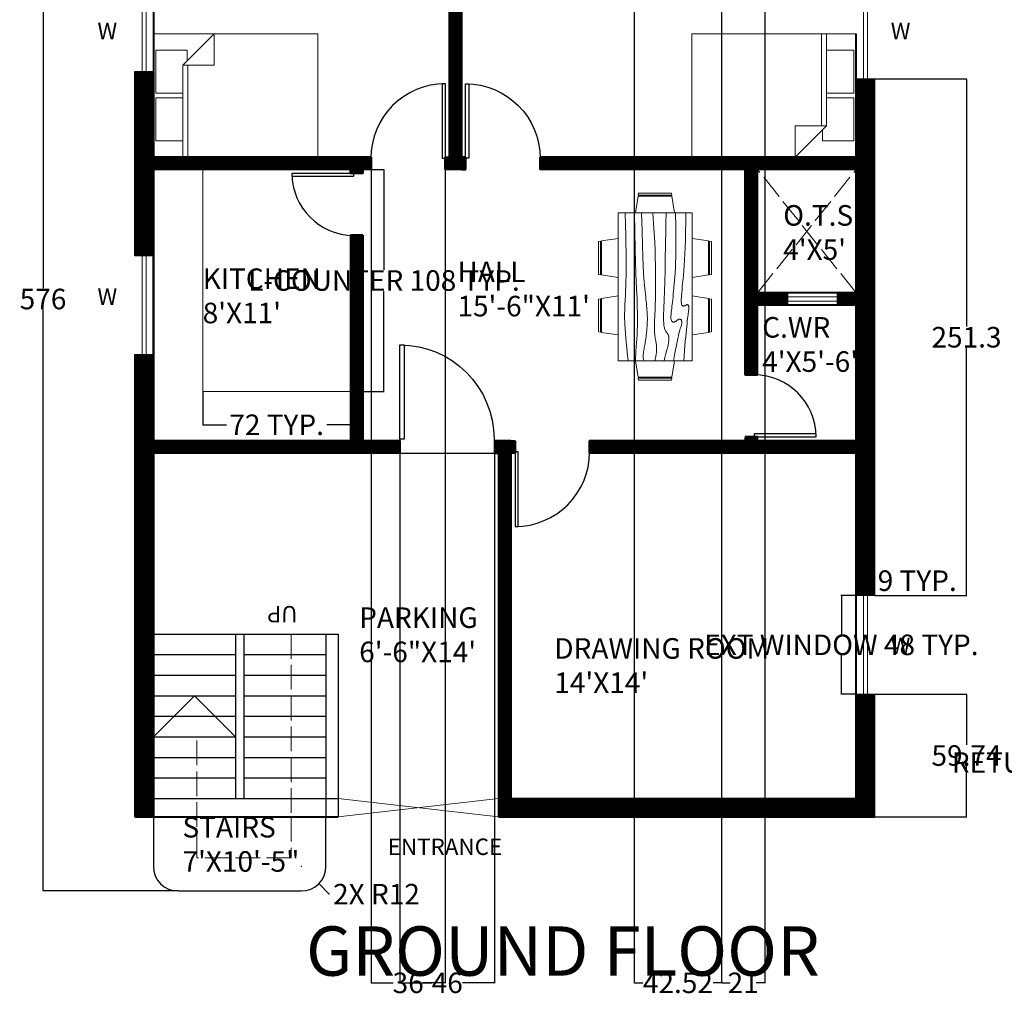
# Model space of a CAD drawing. Units: inches. Extents: x 345 to 1363, y 285 to 1014.
# Tile 1 of 4: x 345 to 824, y 285 to 760. Entities that reach past the tile are written whole.
import ezdxf

# ---------------------------------------------------------------- set-up
doc = ezdxf.new("R2010")
doc.units = ezdxf.units.IN
doc.header["$MEASUREMENT"] = 0
doc.linetypes.add('ACAD_ISO02W100', pattern=[15, 12, -3])
for name, color, linetype, lineweight in [('A-ANNO-DIMS', 2, 'Continuous', 18), ('A-ANNO-SYMB', 3, 'Continuous', 18), ('A-ANNO-TEXT', 7, 'Continuous', 18), ('A-ANNO-TITL', 7, 'Continuous', 35), ('A-AREA-IDEN', 7, 'Continuous', 18), ('A-FLOR-CASE', 8, 'Continuous', 18), ('A-FLOR-OPEN', 8, 'Continuous', 18), ('A-FLOR-OPEN-OVHD', 8, 'ACAD_ISO02W100', 13), ('A-FLOR-STRS', 7, 'Continuous', 25), ('A-FLOR-STRS-PATH', 3, 'ACAD_ISO02W100', 18), ('A-FURN', 9, 'Continuous', 18), ('A-GLAZ', 4, 'Continuous', 18), ('A-WALL', 7, 'Continuous', 40), ('A-WALL-PATT', 252, 'Continuous', 9), ('BED', 9, 'Continuous', 18), ('DOOR', 4, 'Continuous', 25)]:
    doc.layers.add(name, color=color, linetype=linetype, lineweight=lineweight)
doc.styles.get("Standard").update_dxf_attribs({"font": 'arial.ttf'})
doc.dimstyles.get("Standard").update_dxf_attribs({"dimtxt": 10, "dimasz": 0.18, "dimexe": 0.18, "dimexo": 0.0625, "dimgap": 0.09, "dimtad": 0, "dimtih": 1, "dimtoh": 1, "dimdec": 0, "dimzin": 0, "dimdsep": 46, "dimlunit": 3, "dimtxsty": 'Standard', "dimcen": 0.09, "dimadec": 0, "dimazin": 0, "dimtfac": 1, "dimtdec": 0, "dimtofl": 0, "dimtmove": 0, "dimatfit": 3, "dimfxl": 1, "dimtolj": 1, "dimtzin": 0, "dimarcsym": 0})

# ---------------------------------------------------------------- blocks, each defined once
blk = doc.blocks.new('Bed - Queen')
for p, q in [((0, -80.00003), (0, 0)), ((0, 0), (59.99999, 0)), ((59.99999, 0), (59.99999, -80.00003)), ((7.99999, -1.2), (28.79998, -1.2)), ((7.99999, -14.4), (7.99999, -1.2)), ((28.79998, -1.2), (28.79998, -14.4)), ((31.19999, -1.2), (51.99999, -1.2)), ((31.19999, -14.4), (31.19999, -1.2)), ((51.99999, -1.2), (51.99999, -16.4)), ((0, -14.4), (44.8, -14.4)), ((44.8, -16.8), (0, -16.8)), ((59.99999, -29.6), (44.8, -14.4)), ((44.8, -14.4), (44.8, -29.6)), ((51.99999, -16.4), (46.79936, -16.4)), ((44.8, -29.6), (59.99999, -29.6)), ((59.99999, -80.00003), (0, -80.00003))]:
    blk.add_line(p, q)
blk = doc.blocks.new('Dining Set - 36 x 72 in.')
for p, q in [((-22.2343, 26.00059), (-23.4847, 17.99762)), ((-22.2304, 26), (-5.7608, 26)), ((-22, 27.5), (-22.1562, 26.50042)), ((-5.8416, 26.5), (-22.1534, 26.5)), ((-22, 27.5), (-6, 27.5)), ((-5.8437, 26.49966), (-6, 27.5)), ((-4.5152, 17.99762), (-5.7655, 25.99926)), ((5.7657, 26.00059), (4.5153, 17.99762)), ((5.7696, 26), (22.2392, 26)), ((6, 27.5), (5.8438, 26.50042)), ((22.1584, 26.5), (5.8466, 26.5)), ((6, 27.5), (22, 27.5)), ((22.1563, 26.49966), (22, 27.5)), ((23.4848, 17.99762), (22.2345, 25.99926)), ((36, 18), (-36, 18)), ((-36, 18), (-36, -18)), ((36, -18), (36, 18)), ((-45.5, 8), (-44.5004, 8.15617)), ((-45.5, 8), (-45.5, -8)), ((-44.5, -8.15843), (-44.5, 8.15338)), ((-44.0006, 8.23428), (-35.9976, 9.48474)), ((-44, 8.23041), (-44, -8.23915)), ((44.0006, 8.23428), (35.9976, 9.48474)), ((44, 8.23041), (44, -8.23915)), ((44.5, -8.15843), (44.5, 8.15338)), ((45.5, 8), (44.5005, 8.15617)), ((45.5, 8), (45.5, -8)), ((-44.4997, -8.15631), (-45.5, -8)), ((-35.9976, -9.48476), (-43.9993, -8.2345)), ((35.9976, -9.48476), (43.9993, -8.2345)), ((44.4997, -8.15631), (45.5, -8)), ((-36, -18), (36, -18)), ((-22.2343, -26.0006), (-23.4847, -17.99762)), ((-4.5152, -17.99762), (-5.7655, -25.99928)), ((5.7657, -26.0006), (4.5153, -17.99762)), ((23.4848, -17.99762), (22.2345, -25.99928)), ((-22.2304, -26), (-5.7608, -26)), ((-22, -27.5), (-22.1562, -26.50044)), ((-5.8416, -26.5), (-22.1534, -26.5)), ((-22, -27.5), (-6, -27.5)), ((-5.8437, -26.49967), (-6, -27.5)), ((5.7696, -26), (22.2392, -26)), ((6, -27.5), (5.8438, -26.50044)), ((22.1584, -26.5), (5.8466, -26.5)), ((6, -27.5), (22, -27.5)), ((22.1563, -26.49967), (22, -27.5))]:
    blk.add_line(p, q)
for points in [[(-36, 15), (-31.1772, 14.97754), (-26.8079, 14.91406), (-22.8538, 14.81543), (-19.276, 14.6875), (-16.0362, 14.53613), (-13.0957, 14.36718), (-10.4159, 14.18652), (-7.9583, 14), (-5.6904, 13.81315), (-3.6035, 13.63021), (-1.6954, 13.45508), (0.0365, 13.29166), (1.5945, 13.14388), (2.9811, 13.01562), (4.1988, 12.9108), (5.25, 12.83333), (6.1393, 12.78613), (6.8802, 12.76823), (7.4883, 12.77767), (7.9792, 12.8125), (8.3685, 12.87077), (8.6719, 12.95052), (8.9049, 13.0498), (9.0833, 13.16666), (9.2205, 13.29899), (9.3216, 13.44401), (9.3895, 13.59879), (9.4271, 13.76041), (9.4373, 13.92594), (9.4232, 14.09245), (9.3875, 14.257), (9.3333, 14.41666), (9.2638, 14.56917), (9.1836, 14.71484), (9.0975, 14.85465), (9.0104, 14.98958), (8.9272, 15.1206), (8.8529, 15.2487), (8.7922, 15.37483), (8.75, 15.5), (8.7305, 15.62467), (8.7344, 15.74739), (8.7617, 15.86621), (8.8125, 15.97916), (8.8867, 16.08431), (8.9844, 16.17968), (9.1055, 16.26334), (9.25, 16.33333), (9.4189, 16.38802), (9.6172, 16.42708), (9.8506, 16.45052), (10.125, 16.45833), (10.4463, 16.45052), (10.8203, 16.42708), (11.2529, 16.38802), (11.75, 16.33333), (12.3184, 16.26318), (12.9694, 16.17838), (13.7151, 16.07991), (14.5677, 15.96875), (15.5395, 15.84586), (16.6426, 15.71224), (17.8893, 15.56884), (19.2917, 15.41666), (20.859, 15.25667), (22.5879, 15.08984), (24.4721, 14.91715), (26.5052, 14.73958), (28.6809, 14.5581), (30.9929, 14.3737), (33.4347, 14.18733), (36, 14)], [(-36, 10), (-28.9766, 10.14274), (-23.1725, 10.20442), (-18.4241, 10.19775), (-14.5677, 10.13541), (-11.4399, 10.03011), (-8.877, 9.89453), (-6.7154, 9.74137), (-4.7917, 9.58333), (-2.9698, 9.43082), (-1.2246, 9.28515), (0.4415, 9.14534), (2.026, 9.01041), (3.5266, 8.87939), (4.9408, 8.7513), (6.266, 8.62516), (7.5, 8.5), (8.6411, 8.37549), (9.6914, 8.2539), (10.6538, 8.13818), (11.5312, 8.03125), (12.3267, 7.93603), (13.043, 7.85547), (13.6831, 7.79248), (14.25, 7.75), (14.7471, 7.7303), (15.1797, 7.73307), (15.5537, 7.75732), (15.875, 7.80208), (16.1494, 7.86637), (16.3828, 7.94922), (16.5811, 8.04964), (16.75, 8.16666), (16.8944, 8.29915), (17.0143, 8.44531), (17.1089, 8.60319), (17.1771, 8.77083), (17.218, 8.94629), (17.2305, 9.1276), (17.2137, 9.31282), (17.1667, 9.5), (17.0895, 9.6875), (16.987, 9.875), (16.8649, 10.0625), (16.7292, 10.25), (16.5856, 10.4375), (16.4401, 10.625), (16.2985, 10.8125), (16.1667, 11), (16.05, 11.18733), (15.9518, 11.3737), (15.8752, 11.5581), (15.8229, 11.73958), (15.798, 11.91715), (15.8034, 12.08984), (15.842, 12.25667), (15.9167, 12.41666), (16.0295, 12.56836), (16.1784, 12.70833), (16.3605, 12.83268), (16.5729, 12.9375), (16.8127, 13.01888), (17.0768, 13.07291), (17.3625, 13.0957), (17.6667, 13.08333), (17.9894, 13.03312), (18.3418, 12.94726), (18.7382, 12.82918), (19.1927, 12.68229), (19.7195, 12.51001), (20.3327, 12.31575), (21.0465, 12.10294), (21.875, 11.875), (22.8357, 11.63354), (23.959, 11.37304), (25.2786, 11.08618), (26.8282, 10.76562), (28.6414, 10.40405), (30.752, 9.99414), (33.1936, 9.52856), (36, 9)], [(-36, 5.5), (-30.7157, 5.3348), (-26.069, 5.20963), (-21.9946, 5.11767), (-18.4271, 5.05208), (-15.3009, 5.00602), (-12.5508, 4.97265), (-10.1112, 4.94515), (-7.9167, 4.91666), (-5.909, 4.88167), (-4.0586, 4.83984), (-2.3429, 4.79215), (-0.7396, 4.73958), (0.7739, 4.6831), (2.22, 4.6237), (3.6213, 4.56233), (5, 4.5), (6.373, 4.43782), (7.7344, 4.3776), (9.0723, 4.32129), (10.375, 4.27083), (11.6309, 4.22819), (12.8281, 4.19531), (13.9551, 4.17415), (15, 4.16666), (15.954, 4.17448), (16.819, 4.19791), (17.6001, 4.23698), (18.3021, 4.29166), (18.9299, 4.36198), (19.4883, 4.44791), (19.9823, 4.54948), (20.4167, 4.66666), (20.7969, 4.79899), (21.1302, 4.94401), (21.4245, 5.09879), (21.6875, 5.26041), (21.9271, 5.42594), (22.1511, 5.59245), (22.3672, 5.757), (22.5834, 5.91666), (22.8065, 6.06868), (23.0404, 6.21093), (23.2879, 6.34147), (23.5521, 6.45833), (23.8358, 6.55957), (24.142, 6.64323), (24.4735, 6.70735), (24.8334, 6.75), (25.2235, 6.76969), (25.642, 6.76692), (26.0858, 6.74267), (26.5521, 6.69791), (27.0379, 6.63362), (27.5404, 6.55078), (28.0565, 6.45036), (28.5834, 6.33333), (29.1242, 6.19987), (29.7071, 6.04687), (30.3661, 5.87044), (31.1354, 5.66666), (32.0493, 5.43164), (33.142, 5.16146), (34.4475, 4.85221), (36, 4.5)], [(-36, -1), (-30.7915, -0.6591), (-26.0195, -0.38216), (-21.6519, -0.16284), (-17.6563, 0.00521), (-14.0005, 0.12833), (-10.6523, 0.21289), (-7.5796, 0.26522), (-4.75, 0.29166), (-2.134, 0.29793), (0.2878, 0.28711), (2.5317, 0.26163), (4.6146, 0.22396), (6.5529, 0.17651), (8.3633, 0.12174), (10.0623, 0.06209), (11.6667, 0), (13.1899, -0.06201), (14.6341, -0.1211), (15.9982, -0.17432), (17.2813, -0.21875), (18.4823, -0.25147), (19.6003, -0.26953), (20.6343, -0.27002), (21.5834, -0.25), (22.4481, -0.20768), (23.2357, -0.14584), (23.9549, -0.06836), (24.6146, 0.02083), (25.2235, 0.11784), (25.7904, 0.21875), (26.3241, 0.31966), (26.8334, 0.41666), (27.3265, 0.50618), (27.8099, 0.58593), (28.2894, 0.65397), (28.7709, 0.70833), (29.2601, 0.74707), (29.763, 0.76823), (30.2855, 0.76985), (30.8334, 0.75), (31.4088, 0.70784), (31.9994, 0.64713), (32.589, 0.57275), (33.1615, 0.48958), (33.7008, 0.4025), (34.1908, 0.3164), (34.6153, 0.23616), (34.9584, 0.16666), (35.2099, 0.11165), (35.3848, 0.07031), (35.504, 0.04069), (35.5886, 0.02083), (35.6594, 0.00879), (35.7377, 0.0026), (35.8442, 0.00032), (36, 0)], [(-36, -6.5), (-27.1843, -6.31267), (-20.084, -6.1263), (-14.469, -5.9419), (-10.1094, -5.76042), (-6.7752, -5.58285), (-4.2363, -5.41016), (-2.2629, -5.24333), (-0.625, -5.08334), (0.8708, -4.93099), (2.2715, -4.78646), (3.5872, -4.64974), (4.8281, -4.52084), (6.0046, -4.39974), (7.127, -4.28646), (8.2053, -4.18099), (9.25, -4.08334), (10.2705, -3.99382), (11.2734, -3.91407), (12.2647, -3.84603), (13.25, -3.79167), (14.2354, -3.75293), (15.2266, -3.73177), (16.2295, -3.73015), (17.25, -3.75), (18.2912, -3.79248), (19.3451, -3.85547), (20.4009, -3.93604), (21.4479, -4.03125), (22.4754, -4.13819), (23.4727, -4.25391), (24.4289, -4.37549), (25.3334, -4.5), (26.1785, -4.62492), (26.9694, -4.74935), (27.7145, -4.87281), (28.4219, -4.99479), (29.1, -5.11483), (29.7572, -5.23242), (30.4016, -5.34709), (31.0417, -5.45834), (31.6837, -5.56437), (32.3262, -5.65821), (32.9658, -5.73153), (33.599, -5.77604), (34.2224, -5.78345), (34.8327, -5.74545), (35.4264, -5.65373), (36, -5.5)], [(-36, -10), (-26.4022, -9.81299), (-18.4675, -9.62891), (-11.9839, -9.45069), (-6.7396, -9.28125), (-2.5226, -9.12354), (0.8789, -8.98047), (3.6769, -8.85498), (6.0833, -8.75), (8.2767, -8.66765), (10.3021, -8.60677), (12.1712, -8.56543), (13.8958, -8.54167), (15.4876, -8.53353), (16.9583, -8.53907), (18.3197, -8.55632), (19.5834, -8.58334), (20.7616, -8.61841), (21.8685, -8.66081), (22.9188, -8.71004), (23.9271, -8.76563), (24.9081, -8.82707), (25.8763, -8.89388), (26.8465, -8.96558), (27.8334, -9.04167), (28.8474, -9.12118), (29.8828, -9.20117), (30.93, -9.27824), (31.9792, -9.34896), (33.0205, -9.40991), (34.0443, -9.45768), (35.0407, -9.48885), (36, -9.5)], [(-36, -14.5), (-30.0881, -14.33513), (-25.0332, -14.21224), (-20.7312, -14.12647), (-17.0781, -14.07292), (-13.97, -14.04671), (-11.3027, -14.04297), (-8.9724, -14.05681), (-6.875, -14.08334), (-4.9224, -14.11833), (-3.0905, -14.16016), (-1.3709, -14.20785), (0.2448, -14.26042), (1.7647, -14.3169), (3.1973, -14.3763), (4.5507, -14.43767), (5.8333, -14.5), (7.0554, -14.5621), (8.235, -14.62175), (9.3922, -14.67652), (10.5469, -14.72396), (11.7192, -14.76164), (12.929, -14.78711), (14.1965, -14.79794), (15.5417, -14.79167), (16.9933, -14.76424), (18.6152, -14.70508), (20.4804, -14.60197), (22.6615, -14.44271), (25.2312, -14.21509), (28.2624, -13.9069), (31.8277, -13.50594), (36, -13)]]:
    blk.add_lwpolyline(points)
blk = doc.blocks.new('*U8')
for p, q in [((0, 0), (0, -6)), ((-40, 0), (-40, -6))]:
    blk.add_line(p, q)
blk.add_lwpolyline([(0, 0), (0, 40), (-1.75, 40), (-1.75, 0)], close=True)
blk.add_arc((0, 0), 40, 90, 180)
blk = doc.blocks.new('*U9')
for p, q in [((0, 0), (0, 6)), ((40, 0), (40, 6))]:
    blk.add_line(p, q)
blk.add_lwpolyline([(0, 0), (0, -40), (1.75, -40), (1.75, 0)], close=True)
blk.add_arc((0, 0), 40, 270, 360)
blk = doc.blocks.new('WIN-48IN-EXT')
for p, q in [((9, 48), (0, 48)), ((3.5, 0), (3.5, 48)), ((5.5, 0), (5.5, 48)), ((9, 0), (0, 0))]:
    blk.add_line(p, q)
blk = doc.blocks.new('WIN-24IN-VENT')
for p, q in [((0, 24), (6, 24)), ((2, 24), (2, 0)), ((4, 24), (4, 0)), ((0, 0), (6, 0))]:
    blk.add_line(p, q)
blk = doc.blocks.new('KITCHEN-L-COUNTER')
for p in [(0, 108), (72, 0)]:
    blk.add_line(p, (0, 0))
blk = doc.blocks.new('STAIR-RETURN-84IN')
for p, q in [((0, 89), (44, 89)), ((40, 89), (40, 9)), ((44, 89), (44, 9)), ((44, 89), (90, 89)), ((84, 89), (84, 0)), ((90, 89), (90, 0)), ((0, 79), (40, 79)), ((44, 79), (84, 79)), ((0, 69), (40, 69)), ((44, 69), (84, 69)), ((0, 59), (40, 59)), ((44, 59), (84, 59)), ((0, 49), (40, 49)), ((44, 49), (84, 49)), ((0, 39), (40, 39)), ((44, 39), (84, 39)), ((0, 29), (40, 29)), ((44, 29), (84, 29)), ((0, 19), (40, 19)), ((44, 19), (84, 19)), ((0, 9), (90, 9)), ((0, 0), (0, -24)), ((84, -24), (84, 0)), ((12, -36), (72, -36))]:
    blk.add_line(p, q)
for centre, start, end in [((12, -24), 180, 270), ((72, -24), 270, 0)]:
    blk.add_arc(centre, 12, start, end)
blk = doc.blocks.new('STAIR-DIRECTION-ARROWHEAD')
for p, q in [((-20, 0), (0, 20)), ((0, 20), (20, 0)), ((0, 0), (-20, 0)), ((20, 0), (1.17, 0))]:
    blk.add_line(p, q)
blk = doc.blocks.new('*D16')
at = {"layer": 'A-ANNO-DIMS', "color": 0, "lineweight": -2, "transparency": 16777216}
for p, q in [((751.9, 479.51), (744.59, 479.51)), ((744.77, 479.33), (744.77, 460.77)), ((744.77, 431.69), (744.77, 450.24)), ((751.9, 431.51), (744.59, 431.51))]:
    blk.add_line(p, q, dxfattribs=at)
at = {"layer": 'A-ANNO-DIMS', "color": 0, "transparency": 16777216}
for points in [[(744.74, 479.33), (744.8, 479.33), (744.77, 479.51)], [(744.74, 431.69), (744.8, 431.69), (744.77, 431.51)]]:
    blk.add_solid(points, dxfattribs=at)
at = {"layer": 'Defpoints', "color": 0, "transparency": 16777216}
for p in [(744.77, 479.51), (751.97, 479.51), (751.97, 431.51)]:
    blk.add_point(p, dxfattribs=at)
at = {"layer": 'A-ANNO-DIMS', "color": 0, "transparency": 16777216, "insert": (744.77, 455.51), "char_height": 10, "attachment_point": 5}
blk.add_mtext('\\A1;EXT WINDOW 48 TYP.', dxfattribs=at)
blk = doc.blocks.new('*D17')
at = {"layer": 'A-ANNO-DIMS', "color": 0, "lineweight": -2, "transparency": 16777216}
for p, q in [((751.97, 479.57), (751.97, 486.89)), ((752.15, 486.71), (760.79, 486.71)), ((760.97, 479.57), (760.97, 486.89)), ((760.97, 486.71), (761.15, 486.71))]:
    blk.add_line(p, q, dxfattribs=at)
at = {"layer": 'A-ANNO-DIMS', "color": 0, "transparency": 16777216}
for points in [[(752.15, 486.74), (752.15, 486.68), (751.97, 486.71)], [(760.79, 486.74), (760.79, 486.68), (760.97, 486.71)]]:
    blk.add_solid(points, dxfattribs=at)
at = {"layer": 'Defpoints', "color": 0, "transparency": 16777216}
for p in [(760.97, 486.71), (751.97, 479.51), (760.97, 479.51)]:
    blk.add_point(p, dxfattribs=at)
at = {"layer": 'A-ANNO-DIMS', "color": 0, "transparency": 16777216, "insert": (781.69, 486.71), "char_height": 10, "attachment_point": 5}
blk.add_mtext('\\A1;9 TYP.', dxfattribs=at)
blk = doc.blocks.new('*D26')
at = {"layer": 'A-ANNO-DIMS', "color": 0, "lineweight": -2, "transparency": 16777216}
for p, q in [((506.03, 686.76), (522.35, 686.76)), ((522.17, 686.58), (522.17, 638.03)), ((522.17, 578.94), (522.17, 627.5)), ((506.03, 578.76), (522.35, 578.76))]:
    blk.add_line(p, q, dxfattribs=at)
at = {"layer": 'A-ANNO-DIMS', "color": 0, "transparency": 16777216}
for points in [[(522.14, 686.58), (522.2, 686.58), (522.17, 686.76)], [(522.14, 578.94), (522.2, 578.94), (522.17, 578.76)]]:
    blk.add_solid(points, dxfattribs=at)
at = {"layer": 'Defpoints', "color": 0, "transparency": 16777216}
for p in [(505.97, 686.76), (522.17, 686.76), (505.97, 578.76)]:
    blk.add_point(p, dxfattribs=at)
at = {"layer": 'A-ANNO-DIMS', "color": 0, "transparency": 16777216, "insert": (522.17, 632.76), "char_height": 10, "attachment_point": 5}
blk.add_mtext('\\A1;L-COUNTER 108 TYP.', dxfattribs=at)
blk = doc.blocks.new('*D27')
at = {"layer": 'A-ANNO-DIMS', "color": 0, "lineweight": -2, "transparency": 16777216}
for p, q in [((433.97, 578.7), (433.97, 562.38)), ((505.97, 578.7), (505.97, 562.38)), ((434.15, 562.56), (445.58, 562.56)), ((505.79, 562.56), (494.35, 562.56))]:
    blk.add_line(p, q, dxfattribs=at)
at = {"layer": 'A-ANNO-DIMS', "color": 0, "transparency": 16777216}
for points in [[(434.15, 562.59), (434.15, 562.53), (433.97, 562.56)], [(505.79, 562.59), (505.79, 562.53), (505.97, 562.56)]]:
    blk.add_solid(points, dxfattribs=at)
at = {"layer": 'Defpoints', "color": 0, "transparency": 16777216}
for p in [(433.97, 578.76), (505.97, 578.76), (505.97, 562.56)]:
    blk.add_point(p, dxfattribs=at)
at = {"layer": 'A-ANNO-DIMS', "color": 0, "transparency": 16777216, "insert": (469.97, 562.56), "char_height": 10, "attachment_point": 5}
blk.add_mtext('\\A1;72 TYP.', dxfattribs=at)
blk = doc.blocks.new('*D28')
at = {"layer": 'A-ANNO-DIMS', "color": 0, "lineweight": -2, "transparency": 16777216}
for p, q in [((892.32, 460.76), (873.45, 460.76)), ((873.63, 460.58), (873.63, 403.52)), ((873.63, 335.94), (873.63, 393)), ((892.32, 335.76), (873.45, 335.76))]:
    blk.add_line(p, q, dxfattribs=at)
at = {"layer": 'A-ANNO-DIMS', "color": 0, "transparency": 16777216}
for points in [[(873.6, 460.58), (873.66, 460.58), (873.63, 460.76)], [(873.6, 335.94), (873.66, 335.94), (873.63, 335.76)]]:
    blk.add_solid(points, dxfattribs=at)
at = {"layer": 'Defpoints', "color": 0, "transparency": 16777216}
for p in [(873.63, 460.76), (892.38, 460.76), (892.38, 335.76)]:
    blk.add_point(p, dxfattribs=at)
at = {"layer": 'A-ANNO-DIMS', "color": 0, "transparency": 16777216, "insert": (873.63, 398.26), "char_height": 10, "attachment_point": 5}
blk.add_mtext('\\A1;RETURN STAIR 125 TYP.', dxfattribs=at)
blk = doc.blocks.new('*D31')
at = {"layer": 'A-ANNO-DIMS', "color": 0, "lineweight": -2, "transparency": 16777216}
for p, q in [((400.9, 911.76), (356.09, 911.76)), ((356.27, 911.58), (356.27, 628.96)), ((356.27, 335.94), (356.27, 618.57)), ((421.9, 335.76), (356.09, 335.76))]:
    blk.add_line(p, q, dxfattribs=at)
at = {"layer": 'A-ANNO-DIMS', "color": 0, "transparency": 16777216}
for points in [[(356.24, 911.58), (356.3, 911.58), (356.27, 911.76)], [(356.24, 335.94), (356.3, 335.94), (356.27, 335.76)]]:
    blk.add_solid(points, dxfattribs=at)
at = {"layer": 'Defpoints', "color": 0, "transparency": 16777216}
for p in [(356.27, 911.76), (400.97, 911.76), (421.97, 335.76)]:
    blk.add_point(p, dxfattribs=at)
at = {"layer": 'A-ANNO-DIMS', "color": 0, "transparency": 16777216, "insert": (356.27, 623.76), "char_height": 10, "attachment_point": 5}
blk.add_mtext('\\A1;576', dxfattribs=at)
blk = doc.blocks.new('*D37')
at = {"layer": 'A-ANNO-DIMS', "color": 0, "lineweight": -2, "transparency": 16777216}
for p, q in [((761.03, 431.51), (805.85, 431.51)), ((805.67, 431.33), (805.67, 406.83)), ((805.67, 371.94), (805.67, 396.44)), ((761.03, 371.76), (805.85, 371.76))]:
    blk.add_line(p, q, dxfattribs=at)
at = {"layer": 'A-ANNO-DIMS', "color": 0, "transparency": 16777216}
for points in [[(805.64, 431.33), (805.7, 431.33), (805.67, 431.51)], [(805.64, 371.94), (805.7, 371.94), (805.67, 371.76)]]:
    blk.add_solid(points, dxfattribs=at)
at = {"layer": 'Defpoints', "color": 0, "transparency": 16777216}
for p in [(760.97, 431.51), (760.97, 371.76), (805.67, 371.76)]:
    blk.add_point(p, dxfattribs=at)
at = {"layer": 'A-ANNO-DIMS', "color": 0, "transparency": 16777216, "insert": (805.67, 401.64), "char_height": 10, "attachment_point": 5}
blk.add_mtext('\\A1;59.74', dxfattribs=at)
blk = doc.blocks.new('*D38')
at = {"layer": 'A-ANNO-DIMS', "color": 0, "lineweight": -2, "transparency": 16777216}
for p, q in [((761.03, 730.81), (805.85, 730.81)), ((805.67, 730.63), (805.67, 610.36)), ((805.67, 479.69), (805.67, 599.96)), ((761.03, 479.51), (805.85, 479.51))]:
    blk.add_line(p, q, dxfattribs=at)
at = {"layer": 'A-ANNO-DIMS', "color": 0, "transparency": 16777216}
for points in [[(805.64, 730.63), (805.7, 730.63), (805.67, 730.81)], [(805.64, 479.69), (805.7, 479.69), (805.67, 479.51)]]:
    blk.add_solid(points, dxfattribs=at)
at = {"layer": 'Defpoints', "color": 0, "transparency": 16777216}
for p in [(760.97, 730.81), (760.97, 479.51), (805.67, 479.51)]:
    blk.add_point(p, dxfattribs=at)
at = {"layer": 'A-ANNO-DIMS', "color": 0, "transparency": 16777216, "insert": (805.67, 605.16), "char_height": 10, "attachment_point": 5}
blk.add_mtext('\\A1;251.3', dxfattribs=at)
blk = doc.blocks.new('*D39')
at = {"layer": 'A-ANNO-DIMS', "color": 0, "lineweight": -2, "transparency": 16777216}
for p, q in [((529.97, 548.7), (529.97, 290.88)), ((575.97, 548.7), (575.97, 290.88)), ((530.15, 291.06), (545.52, 291.06)), ((575.79, 291.06), (560.42, 291.06))]:
    blk.add_line(p, q, dxfattribs=at)
at = {"layer": 'A-ANNO-DIMS', "color": 0, "transparency": 16777216}
for points in [[(530.15, 291.09), (530.15, 291.03), (529.97, 291.06)], [(575.79, 291.09), (575.79, 291.03), (575.97, 291.06)]]:
    blk.add_solid(points, dxfattribs=at)
at = {"layer": 'Defpoints', "color": 0, "transparency": 16777216}
for p in [(529.97, 548.76), (575.97, 548.76), (575.97, 291.06)]:
    blk.add_point(p, dxfattribs=at)
at = {"layer": 'A-ANNO-DIMS', "color": 0, "transparency": 16777216, "insert": (552.97, 291.06), "char_height": 10, "attachment_point": 5}
blk.add_mtext('\\A1;46', dxfattribs=at)
blk = doc.blocks.new('*D40')
at = {"layer": 'A-ANNO-DIMS', "color": 0, "lineweight": -2, "transparency": 16777216}
for p, q in [((515.97, 686.7), (515.97, 290.88)), ((551.97, 686.7), (551.97, 290.88)), ((516.15, 291.06), (526.72, 291.06)), ((551.79, 291.06), (541.21, 291.06))]:
    blk.add_line(p, q, dxfattribs=at)
at = {"layer": 'A-ANNO-DIMS', "color": 0, "transparency": 16777216}
for points in [[(516.15, 291.09), (516.15, 291.03), (515.97, 291.06)], [(551.79, 291.09), (551.79, 291.03), (551.97, 291.06)]]:
    blk.add_solid(points, dxfattribs=at)
at = {"layer": 'Defpoints', "color": 0, "transparency": 16777216}
for p in [(515.97, 686.76), (551.97, 686.76), (551.97, 291.06)]:
    blk.add_point(p, dxfattribs=at)
at = {"layer": 'A-ANNO-DIMS', "color": 0, "transparency": 16777216, "insert": (533.97, 291.06), "char_height": 10, "attachment_point": 5}
blk.add_mtext('\\A1;36', dxfattribs=at)
blk = doc.blocks.new('*D43')
at = {"layer": 'A-ANNO-DIMS', "color": 0, "lineweight": -2, "transparency": 16777216}
for p, q in [((643.97, 902.7), (643.97, 290.88)), ((686.49, 894.7), (686.49, 290.88)), ((644.15, 291.06), (648.11, 291.06)), ((686.31, 291.06), (682.34, 291.06))]:
    blk.add_line(p, q, dxfattribs=at)
at = {"layer": 'A-ANNO-DIMS', "color": 0, "transparency": 16777216}
for points in [[(644.15, 291.09), (644.15, 291.03), (643.97, 291.06)], [(686.31, 291.09), (686.31, 291.03), (686.49, 291.06)]]:
    blk.add_solid(points, dxfattribs=at)
at = {"layer": 'Defpoints', "color": 0, "transparency": 16777216}
for p in [(643.97, 902.76), (686.49, 894.76), (686.49, 291.06)]:
    blk.add_point(p, dxfattribs=at)
at = {"layer": 'A-ANNO-DIMS', "color": 0, "transparency": 16777216, "insert": (665.23, 291.06), "char_height": 10, "attachment_point": 5}
blk.add_mtext('\\A1;42.52', dxfattribs=at)
blk = doc.blocks.new('*D44')
at = {"layer": 'A-ANNO-DIMS', "color": 0, "lineweight": -2, "transparency": 16777216}
for p, q in [((686.49, 894.7), (686.49, 290.88)), ((707.49, 894.7), (707.49, 290.88)), ((686.67, 291.06), (690.61, 291.06)), ((707.31, 291.06), (703.36, 291.06))]:
    blk.add_line(p, q, dxfattribs=at)
at = {"layer": 'A-ANNO-DIMS', "color": 0, "transparency": 16777216}
for points in [[(686.67, 291.09), (686.67, 291.03), (686.49, 291.06)], [(707.31, 291.09), (707.31, 291.03), (707.49, 291.06)]]:
    blk.add_solid(points, dxfattribs=at)
at = {"layer": 'Defpoints', "color": 0, "transparency": 16777216}
for p in [(686.49, 894.76), (707.49, 894.76), (707.49, 291.06)]:
    blk.add_point(p, dxfattribs=at)
at = {"layer": 'A-ANNO-DIMS', "color": 0, "transparency": 16777216, "insert": (696.99, 291.06), "char_height": 10, "attachment_point": 5}
blk.add_mtext('\\A1;21', dxfattribs=at)
blk = doc.blocks.new('*D47')
at = {"layer": 'A-ANNO-DIMS', "color": 0, "lineweight": -2, "transparency": 16777216}
for p, q in [((481.88, 347.76), (482.06, 347.76)), ((481.97, 347.67), (481.97, 347.85)), ((495.54, 334.19), (490.58, 339.15)), ((495.72, 334.19), (495.54, 334.19))]:
    blk.add_line(p, q, dxfattribs=at)
at = {"layer": 'A-ANNO-DIMS', "color": 0, "transparency": 16777216}
blk.add_solid([(490.6, 339.17), (490.56, 339.13), (490.45, 339.28)], dxfattribs=at)
at = {"layer": 'Defpoints', "color": 0, "transparency": 16777216}
for p in [(481.97, 347.76), (490.45, 339.28)]:
    blk.add_point(p, dxfattribs=at)
at = {"layer": 'A-ANNO-DIMS', "color": 0, "transparency": 16777216, "insert": (518.54, 334.19), "char_height": 10, "attachment_point": 5}
blk.add_mtext('\\A1;2X R12', dxfattribs=at)

msp = doc.modelspace()

# ---------------------------------------------------------------- hatches: boundary and pattern name
at = {"layer": 'A-WALL-PATT'}
h = msp.add_hatch(dxfattribs=at)
h.set_pattern_fill('ANSI31', color=256)
h.paths.add_polyline_path([(760.967, 730.806), (751.967, 730.806), (751.967, 692.764), (671.967, 692.764), (598.143, 692.764), (598.143, 686.764), (697.967, 686.764), (697.967, 586.835), (702.4, 586.835, -0.0130342), (703.967, 586.794), (703.967, 686.764), (751.967, 686.764), (751.967, 626.764), (742.74, 626.764), (742.74, 620.764), (751.967, 620.764), (751.967, 554.764), (703.967, 554.764), (703.967, 556.764), (702.4, 556.764), (697.967, 556.764), (697.967, 554.764), (622.228, 554.764), (622.228, 548.764), (751.967, 548.764), (751.967, 479.508), (760.967, 479.508)])
h.paths.add_polyline_path([(760.967, 431.508), (751.967, 431.508), (751.967, 380.764), (583.967, 380.764), (583.967, 548.764), (585.967, 548.764), (585.967, 549.325), (585.967, 554.764), (583.967, 554.764), (577.967, 554.764), (575.967, 554.764), (575.967, 548.764), (577.967, 548.764), (577.967, 371.764), (760.967, 371.764)])
h.paths.add_polyline_path([(409.967, 548.764), (529.967, 548.764), (529.967, 554.764), (511.967, 554.764), (511.967, 654.693), (507.456, 654.693, -0.0123881), (505.967, 654.73), (505.967, 554.764), (409.967, 554.764), (409.967, 596.764), (400.967, 596.764), (400.967, 371.764), (409.967, 371.764)])
h.paths.add_polyline_path([(409.967, 686.764), (505.967, 686.764), (505.967, 684.764), (507.456, 684.764), (511.967, 684.764), (511.967, 686.764), (515.791, 686.764), (515.791, 692.764), (409.967, 692.764), (409.967, 734.364), (400.967, 734.364), (400.967, 644.764), (409.967, 644.764)])
h.paths.add_polyline_path([(559.967, 824.764), (561.801, 824.764), (561.801, 829.275), (561.801, 830.764), (559.967, 830.764), (559.967, 902.764), (637.967, 902.764), (637.967, 878.764), (643.967, 878.764), (643.967, 902.764), (751.967, 902.764), (751.967, 830.764), (749.967, 830.764), (749.967, 829.275), (749.967, 824.764), (751.967, 824.764), (751.967, 778.806), (760.967, 778.806), (760.967, 911.764), (400.967, 911.764), (400.967, 782.364), (409.967, 782.364), (409.967, 824.764), (411.967, 824.764), (411.967, 829.275), (411.967, 830.764), (409.967, 830.764), (409.967, 902.764), (553.967, 902.764), (553.967, 830.764), (552.038, 830.764), (552.038, 829.275), (552.038, 824.764), (553.967, 824.764), (553.967, 692.764), (552.052, 692.764), (552.052, 692.203), (552.052, 686.764), (553.967, 686.764), (559.967, 686.764), (561.882, 686.764), (561.882, 692.764), (559.967, 692.764)])
h.paths.add_polyline_path([(718.74, 626.764), (703.967, 626.764), (703.967, 620.764), (718.74, 620.764)], flags=17)
h.paths.add_polyline_path([(892.382, 824.764), (894.382, 824.764), (894.382, 829.275), (894.382, 830.764), (892.382, 830.764), (892.382, 902.764), (1036.382, 902.764), (1036.382, 830.764), (1034.453, 830.764), (1034.453, 829.275), (1034.453, 824.764), (1036.382, 824.764), (1036.382, 692.764), (1034.467, 692.764), (1034.467, 692.203), (1034.467, 686.764), (1036.382, 686.764), (1042.382, 686.764), (1044.297, 686.764), (1044.297, 692.764), (1042.382, 692.764), (1042.382, 824.764), (1044.216, 824.764), (1044.216, 829.275), (1044.216, 830.764), (1042.382, 830.764), (1042.382, 902.764), (1120.382, 902.764), (1120.382, 878.764), (1126.382, 878.764), (1126.382, 902.764), (1234.382, 902.764), (1234.382, 830.764), (1232.382, 830.764), (1232.382, 829.275), (1232.382, 824.764), (1234.382, 824.764), (1234.382, 778.806), (1243.382, 778.806), (1243.382, 911.764), (883.382, 911.764), (883.382, 782.364), (892.382, 782.364)])
h.paths.add_polyline_path([(1243.382, 730.806), (1234.382, 730.806), (1234.382, 692.764), (1080.382, 692.764), (1080.382, 686.764), (1180.382, 686.764), (1180.382, 586.764), (1186.382, 586.764), (1186.382, 686.764), (1234.382, 686.764), (1234.382, 626.764), (1225.155, 626.764), (1225.155, 620.764), (1234.382, 620.764), (1234.382, 554.764), (1186.382, 554.764), (1186.382, 556.764), (1180.382, 556.764), (1180.382, 554.764), (1104.382, 554.764), (1104.382, 548.764), (1234.382, 548.764), (1234.382, 479.508), (1243.382, 479.508)])
h.paths.add_polyline_path([(892.382, 686.764), (988.382, 686.764), (988.382, 684.764), (989.871, 684.764), (994.382, 684.764), (994.382, 686.764), (998.206, 686.764), (998.206, 692.203, -0.0038664), (998.21, 692.764), (892.382, 692.764), (892.382, 734.364), (883.382, 734.364), (883.382, 644.764), (892.382, 644.764)])
h.paths.add_polyline_path([(1066.382, 548.764), (1068.382, 548.764), (1068.382, 554.764), (1066.382, 554.764), (1060.382, 554.764), (1058.382, 554.764), (1058.382, 548.764), (1060.382, 548.764), (1060.382, 371.764), (1243.382, 371.764), (1243.382, 431.508), (1234.382, 431.508), (1234.382, 380.764), (1154.382, 380.764), (1066.382, 380.764)])
h.paths.add_polyline_path([(1201.155, 626.764), (1186.382, 626.764), (1186.382, 620.764), (1201.155, 620.764)], flags=17)
h.paths.add_polyline_path([(892.382, 596.764), (883.382, 596.764), (883.382, 371.764), (892.382, 371.764), (892.382, 548.764), (1012.382, 548.764), (1012.382, 554.764), (994.382, 554.764), (994.382, 654.764), (988.382, 654.764), (988.382, 554.764), (892.382, 554.764)])

# ---------------------------------------------------------------- linework, layer by layer
at = {"layer": 'A-FLOR-OPEN'}
for p, q in [((499.967, 380.764), (577.967, 371.764)), ((577.967, 380.764), (499.967, 371.764))]:
    msp.add_line(p, q, dxfattribs=at)
at = {"layer": 'A-FLOR-OPEN-OVHD'}
for p, q in [((703.967, 626.764), (751.967, 686.764)), ((751.967, 626.764), (703.967, 686.764))]:
    msp.add_line(p, q, dxfattribs=at)
at = {"layer": 'A-FLOR-STRS-PATH'}
for p, q in [((476.967, 460.764), (476.967, 371.764)), ((431.136, 351.941), (431.136, 410.764)), ((476.967, 371.764), (476.967, 351.941)), ((476.967, 351.941), (431.136, 351.941))]:
    msp.add_line(p, q, dxfattribs=at)
at = {"layer": 'A-WALL'}
for p, q in [((409.967, 824.764), (409.967, 692.764)), ((553.967, 824.764), (553.967, 692.764)), ((559.967, 824.764), (559.967, 692.764)), ((751.967, 692.764), (751.967, 752.764)), ((400.967, 734.364), (400.967, 644.764)), ((760.967, 479.508), (760.967, 730.806)), ((515.967, 692.764), (409.967, 692.764)), ((515.967, 692.764), (515.967, 686.764)), ((551.967, 686.764), (551.967, 692.764)), ((551.967, 692.764), (553.967, 692.764)), ((561.967, 692.764), (559.967, 692.764)), ((561.967, 686.764), (561.967, 692.764)), ((751.967, 692.764), (597.967, 692.764)), ((597.967, 692.764), (597.967, 686.764)), ((505.967, 686.764), (409.967, 686.764)), ((409.967, 686.764), (409.967, 554.764)), ((409.967, 554.764), (409.967, 686.764)), ((505.967, 684.764), (505.967, 686.764)), ((511.967, 686.764), (511.967, 684.764)), ((515.967, 686.764), (511.967, 686.764)), ((553.967, 686.764), (551.967, 686.764)), ((559.967, 686.764), (553.967, 686.764)), ((559.967, 686.764), (561.967, 686.764)), ((697.967, 686.764), (597.967, 686.764)), ((697.967, 586.764), (697.967, 686.764)), ((751.967, 686.764), (703.967, 686.764)), ((703.967, 586.764), (703.967, 686.764)), ((751.967, 626.764), (751.967, 686.764)), ((511.967, 684.764), (505.967, 684.764)), ((505.967, 654.764), (505.967, 554.764)), ((511.967, 654.764), (505.967, 654.764)), ((511.967, 654.764), (511.967, 554.764)), ((751.967, 626.764), (703.967, 626.764)), ((751.967, 620.764), (703.967, 620.764)), ((751.967, 554.764), (751.967, 620.764)), ((400.967, 596.764), (400.967, 371.764)), ((703.967, 586.764), (697.967, 586.764)), ((703.967, 556.764), (697.967, 556.764)), ((697.967, 556.764), (697.967, 554.764)), ((703.967, 554.764), (703.967, 556.764)), ((505.967, 554.764), (409.967, 554.764)), ((529.967, 554.764), (511.967, 554.764)), ((529.967, 554.764), (529.967, 548.764)), ((577.967, 554.764), (575.967, 554.764)), ((575.967, 554.764), (575.967, 548.764)), ((583.967, 554.764), (577.967, 554.764)), ((583.967, 554.764), (585.967, 554.764)), ((585.967, 554.764), (585.967, 548.764)), ((697.967, 554.764), (621.967, 554.764)), ((621.967, 554.764), (621.967, 548.764)), ((751.967, 554.764), (703.967, 554.764)), ((529.967, 548.764), (409.967, 548.764)), ((409.967, 548.764), (409.967, 371.764)), ((575.967, 548.764), (577.967, 548.764)), ((577.967, 548.764), (577.967, 371.764)), ((583.967, 548.764), (583.967, 380.764)), ((585.967, 548.764), (583.967, 548.764)), ((751.967, 548.764), (621.967, 548.764)), ((751.967, 380.764), (751.967, 548.764)), ((760.967, 371.764), (760.967, 431.508)), ((583.967, 380.764), (751.967, 380.764)), ((400.967, 371.764), (499.967, 371.764)), ((577.967, 371.764), (760.967, 371.764))]:
    msp.add_line(p, q, dxfattribs=at)
at = {"layer": 'DOOR'}
msp.add_line((529.967, 548.764), (575.753, 548.764), dxfattribs=at)

# ---------------------------------------------------------------- block references
at = {"layer": 'A-ANNO-SYMB'}
msp.add_blockref('STAIR-DIRECTION-ARROWHEAD', (429.967, 410.764), dxfattribs=at)
at = {"layer": 'A-FLOR-CASE'}
msp.add_blockref('KITCHEN-L-COUNTER', (433.967, 578.764), dxfattribs=at)
at = {"layer": 'A-FLOR-STRS'}
msp.add_blockref('STAIR-RETURN-84IN', (409.967, 371.764), dxfattribs=at)
at = {"layer": 'A-FURN', "rotation": 270}
msp.add_blockref('Dining Set - 36 x 72 in.', (654.087, 629.745), dxfattribs=at)
at = {"layer": 'A-GLAZ'}
for p in [(400.967, 734.364), (751.967, 730.806), (400.967, 596.764), (751.967, 431.508)]:
    msp.add_blockref('WIN-48IN-EXT', p, dxfattribs=at)
at = {"layer": 'A-GLAZ', "rotation": 90.00000000000043}
msp.add_blockref('WIN-24IN-VENT', (742.74, 620.764), dxfattribs=at)
at = {"layer": 'BED'}
for p, rotation in [((409.967, 692.764), 89.99999999999999), ((751.967, 752.764), 270)]:
    msp.add_blockref('Bed - Queen', p, dxfattribs=dict(at, rotation=rotation))
at = {"layer": 'DOOR', "yscale": 0.9065366308444065, "zscale": 0.9065366308444065}
for p, xscale in [((552.052, 692.203), 0.9065366308444065), ((561.882, 692.203), -0.9065366308444065)]:
    msp.add_blockref('*U8', p, dxfattribs=dict(at, xscale=xscale))
at = {"layer": 'DOOR'}
for name, p, xscale, yscale, zscale, rotation in [('*U8', (507.456, 684.764), 0.7517678943473934, 0.7517678943473934, 0.7517678943473934, 90), ('*U9', (529.967, 555.632), -1.144664294745111, 1.144664294745111, 1.144664294745111, 180), ('*U9', (702.4, 556.764), 0.7517678943473934, 0.7517678943473934, 0.7517678943473934, 90), ('*U8', (585.967, 549.325), 0.9065366308444065, 0.9065366308444065, 0.9065366308444065, 180)]:
    msp.add_blockref(name, p, dxfattribs=dict(at, xscale=xscale, yscale=yscale, zscale=zscale, rotation=rotation))

# ---------------------------------------------------------------- texts
at = {"layer": 'A-ANNO-TEXT', "char_height": 8, "attachment_point": 1}
for s, insert in [('W', (382.757, 758.158)), ('W', (768.804, 758.158)), ('W', (382.757, 628.908)), ('W', (768.804, 459.059)), ('ENTRANCE', (524, 361.252))]:
    msp.add_mtext_dynamic_manual_height_columns(s, width=42.31972, gutter_width=1, heights=[0], dxfattribs=dict(at, insert=insert))
at = {"layer": 'A-ANNO-TEXT', "insert": (480.089, 466.387), "char_height": 8, "attachment_point": 1, "rotation": 180}
msp.add_mtext_dynamic_manual_height_columns('UP', width=42.31972, gutter_width=1, heights=[0], dxfattribs=at)
at = {"layer": 'A-ANNO-TITL', "insert": (484.244, 318.524), "char_height": 24, "attachment_point": 1}
msp.add_mtext_dynamic_manual_height_columns('{\\fTimes New Roman|b0|i0|c0|p18;GROUND FLOOR}', width=334.9459, gutter_width=1, heights=[0], dxfattribs=at)
at = {"layer": 'A-AREA-IDEN', "char_height": 10, "attachment_point": 1}
for s, insert in [("O.T.S\\P4'X5'", (716.492, 669.434)), ("KITCHEN\\P8'X11'", (433.967, 638.621)), ('HALL\\P15\'-6"X11\'', (557.944, 641.974)), ('C.WR\\P4\'X5\'-6"', (706.247, 614.976)), ('PARKING\\P6\'-6"X14\'', (510.126, 473.729)), ("DRAWING ROOM\\P14'X14'", (605.075, 458.74)), ('STAIRS\\P7\'X10\'-5"', (424.133, 371.764))]:
    msp.add_mtext_dynamic_manual_height_columns(s, width=177.75817, gutter_width=1, heights=[0], dxfattribs=dict(at, insert=insert))

# ---------------------------------------------------------------- dimensions: what is measured, and where the dimension line sits
at = {"layer": 'A-ANNO-DIMS'}
for base, p1, p2, angle, override, picture, middle in [((356.267, 911.764), (421.967, 335.764), (400.967, 911.764), 90, {"dimdec": 0, "dimlfac": 1, "dimrnd": 0, "dimzin": 0, "dimdsep": 46, "dimlunit": 2}, '*D31', (356.267, 623.764)), ((805.667, 479.508), (760.967, 730.806), (760.967, 479.508), 270, {"dimdec": 1, "dimlfac": 1, "dimrnd": 0, "dimzin": 0, "dimdsep": 46, "dimlunit": 2}, '*D38', (805.667, 605.157)), ((805.667, 371.764), (760.967, 431.508), (760.967, 371.764), 270, {"dimdec": 2, "dimlfac": 1, "dimrnd": 0, "dimzin": 0, "dimdsep": 46, "dimlunit": 2}, '*D37', (805.667, 401.636))]:
    dim = msp.add_linear_dim(base=base, p1=p1, p2=p2, angle=angle, dimstyle='Standard', override=override, dxfattribs=at)
    dim.commit()
    dim.dimension.update_dxf_attribs({"geometry": picture, "text_midpoint": middle})
for base, p1, p2, override, picture, middle in [((686.486, 291.064), (643.967, 902.764), (686.486, 894.764), {"dimdec": 2, "dimlfac": 1, "dimrnd": 0, "dimzin": 0, "dimdsep": 46, "dimlunit": 2}, '*D43', (665.226, 291.064)), ((707.486, 291.064), (686.486, 894.764), (707.486, 894.764), {"dimdec": 0, "dimlfac": 1, "dimrnd": 0, "dimzin": 0, "dimdsep": 46, "dimlunit": 2}, '*D44', (696.986, 291.064)), ((551.967, 291.064), (515.967, 686.764), (551.967, 686.764), {"dimdec": 0, "dimlfac": 1, "dimrnd": 0, "dimzin": 0, "dimdsep": 46, "dimlunit": 2}, '*D40', (533.967, 291.064)), ((575.967, 291.064), (529.967, 548.764), (575.967, 548.764), {"dimdec": 0, "dimlfac": 1, "dimrnd": 0, "dimzin": 0, "dimdsep": 46, "dimlunit": 2}, '*D39', (552.967, 291.064))]:
    dim = msp.add_linear_dim(base=base, p1=p1, p2=p2, dimstyle='Standard', override=override, dxfattribs=at)
    dim.commit()
    dim.dimension.update_dxf_attribs({"geometry": picture, "text_midpoint": middle})
for base, p1, p2, text, picture, middle in [((522.167, 686.764), (505.967, 578.764), (505.967, 686.764), 'L-COUNTER <> TYP.', '*D26', (522.167, 632.764)), ((744.767, 479.508), (751.967, 431.508), (751.967, 479.508), 'EXT WINDOW <> TYP.', '*D16', (744.767, 455.508)), ((873.632, 460.764), (892.382, 335.764), (892.382, 460.764), 'RETURN STAIR <> TYP.', '*D28', (873.632, 398.264))]:
    dim = msp.add_linear_dim(base=base, p1=p1, p2=p2, angle=90, text=text, dimstyle='Standard', override={"dimdec": 0, "dimlfac": 1, "dimrnd": 0, "dimzin": 0, "dimdsep": 46, "dimlunit": 2}, dxfattribs=at)
    dim.commit()
    dim.dimension.update_dxf_attribs({"geometry": picture, "text_midpoint": middle})
for base, p1, p2, picture, middle in [((505.967, 562.564), (433.967, 578.764), (505.967, 578.764), '*D27', (469.967, 562.564)), ((760.967, 486.708), (751.967, 479.508), (760.967, 479.508), '*D17', (781.69, 486.708))]:
    dim = msp.add_linear_dim(base=base, p1=p1, p2=p2, text='<> TYP.', dimstyle='Standard', override={"dimdec": 0, "dimlfac": 1, "dimrnd": 0, "dimzin": 0, "dimdsep": 46, "dimlunit": 2}, dxfattribs=at)
    dim.commit()
    dim.dimension.update_dxf_attribs({"geometry": picture, "text_midpoint": middle})
dim = msp.add_radius_dim(center=(481.967, 347.764), mpoint=(490.452, 339.279), text='2X <>', dimstyle='Standard', override={"dimdec": 0, "dimlfac": 1, "dimrnd": 0, "dimzin": 0, "dimdsep": 46, "dimlunit": 2}, dxfattribs=at)
dim.commit()
dim.dimension.update_dxf_attribs({"geometry": '*D47', "text_midpoint": (518.538, 334.188), "dimtype": 164})

doc.saveas('drawing.dxf')
